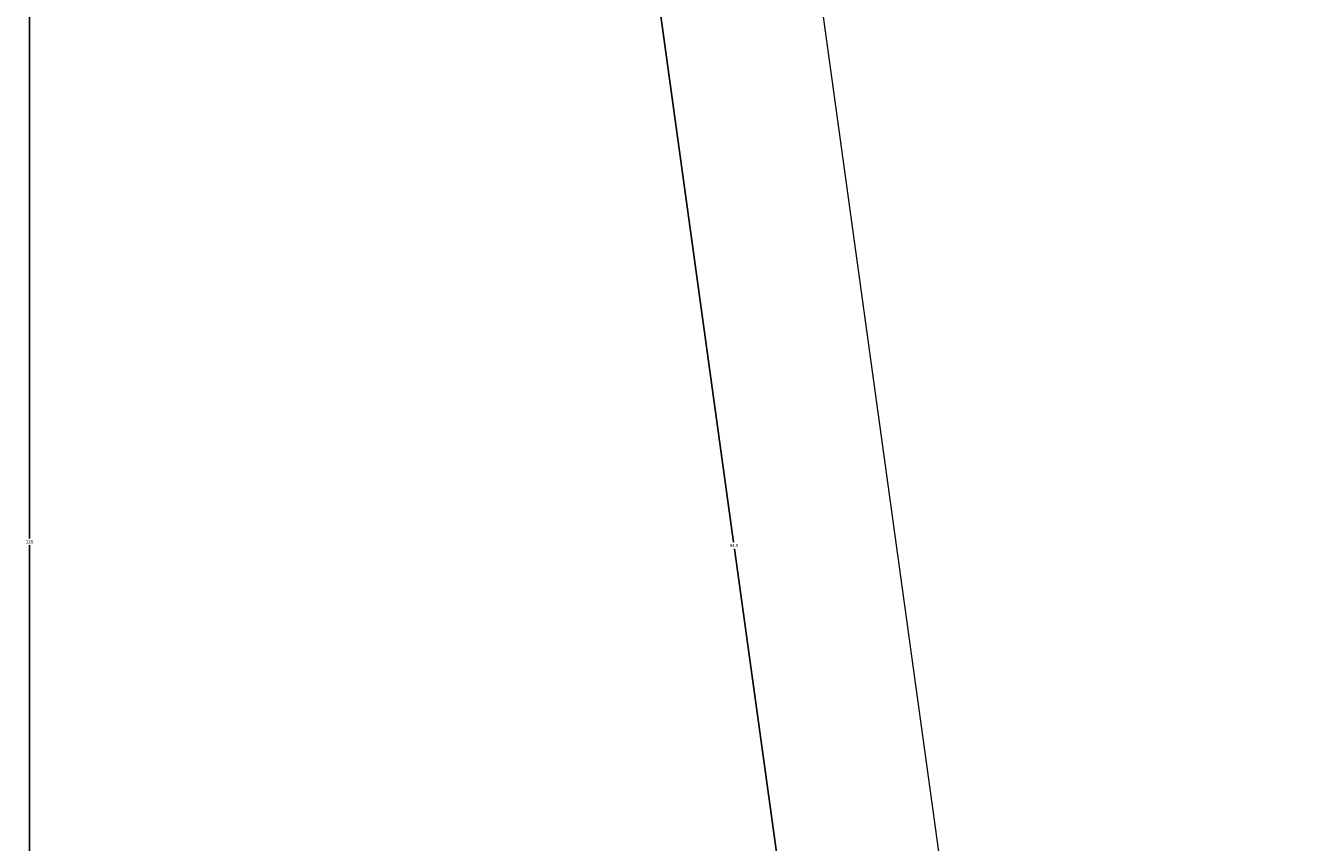
# Model space of a CAD drawing. Units: millimetres. Extents: x -9 to 135, y -119 to 27.
# Tile 3 of 12: x -9 to 62, y -63 to -18. Entities that reach past the tile are written whole.
import ezdxf

# ---------------------------------------------------------------- set-up
doc = ezdxf.new("R2010")
doc.units = ezdxf.units.MM
doc.layers.add('M-CONS', color=8, linetype='Continuous', lineweight=18)
doc.layers.add('M-DIMS', color=2, linetype='Continuous', lineweight=18)
doc.styles.get("Standard").update_dxf_attribs({"font": 'arial.ttf'})
doc.dimstyles.get("Standard").update_dxf_attribs({"dimtxt": 0.18, "dimasz": 0.18, "dimexe": 0.18, "dimexo": 0.0625, "dimgap": 0.09, "dimtad": 0, "dimtih": 1, "dimtoh": 1, "dimdec": 4, "dimzin": 0, "dimdsep": 46, "dimtxsty": 'Standard', "dimcen": 0.09, "dimadec": 0, "dimazin": 0, "dimtfac": 1, "dimtdec": 4, "dimtofl": 0, "dimtmove": 0, "dimatfit": 3, "dimfxl": 1, "dimtolj": 1, "dimtzin": 0, "dimarcsym": 0})

# ---------------------------------------------------------------- blocks, each defined once
blk = doc.blocks.new('*D3')
at = {"layer": 'Defpoints', "color": 0, "transparency": 16777216}
for p in [(0, 17.733), (-8.8, -110.267), (63, -110.267)]:
    blk.add_point(p, dxfattribs=at)
at = {"layer": 'M-DIMS', "color": 0, "lineweight": -2, "transparency": 16777216}
for p, q in [((-0.062, 17.733), (-8.98, 17.733)), ((-8.8, 17.553), (-8.8, -46.085)), ((-8.8, -110.087), (-8.8, -46.449)), ((62.938, -110.267), (-8.98, -110.267))]:
    blk.add_line(p, q, dxfattribs=at)
at = {"layer": 'M-DIMS', "color": 0, "transparency": 16777216}
for points in [[(-8.83, 17.553), (-8.77, 17.553), (-8.8, 17.733)], [(-8.83, -110.087), (-8.77, -110.087), (-8.8, -110.267)]]:
    blk.add_solid(points, dxfattribs=at)
at = {"layer": 'M-DIMS', "color": 0, "transparency": 16777216, "insert": (-8.8, -46.267), "char_height": 0.18, "attachment_point": 5}
blk.add_mtext('\\A1;128', dxfattribs=at)
blk = doc.blocks.new('*D14')
at = {"layer": 'Defpoints', "color": 0, "transparency": 16777216}
for p in [(32, 1.733), (23.283, 0.528), (45, -92.267)]:
    blk.add_point(p, dxfattribs=at)
at = {"layer": 'M-DIMS', "color": 0, "lineweight": -2, "transparency": 16777216}
for p, q in [((31.938, 1.725), (23.105, 0.503)), ((23.308, 0.349), (29.758, -46.29)), ((36.258, -93.294), (29.808, -46.654)), ((44.938, -92.275), (36.105, -93.497))]:
    blk.add_line(p, q, dxfattribs=at)
at = {"layer": 'M-DIMS', "color": 0, "transparency": 16777216}
for points in [[(23.337, 0.353), (23.278, 0.345), (23.283, 0.528)], [(36.288, -93.29), (36.229, -93.298), (36.283, -93.472)]]:
    blk.add_solid(points, dxfattribs=at)
at = {"layer": 'M-DIMS', "color": 0, "transparency": 16777216, "insert": (29.783, -46.472), "char_height": 0.18, "attachment_point": 5}
blk.add_mtext('\\A1;94.9', dxfattribs=at)

msp = doc.modelspace()

# ---------------------------------------------------------------- linework, layer by layer
at = {"layer": 'M-CONS'}
msp.add_line((32, 1.733, 115.129), (45, -92.267, 115.129), dxfattribs=at)

# ---------------------------------------------------------------- dimensions: what is measured, and where the dimension line sits
at = {"layer": 'M-DIMS'}
for base, p1, p2, angle, override, picture, middle in [((-8.8, -110.267), (0, 17.733), (63, -110.267), 90, {"dimdec": 0, "dimlfac": 1, "dimrnd": 0, "dimzin": 0, "dimdsep": 46, "dimlunit": 2}, '*D3', (-8.8, -46.267)), ((23.283, 0.528), (45, -92.267), (32, 1.733), 97.87394, {"dimdec": 1, "dimlfac": 1, "dimrnd": 0, "dimzin": 0, "dimdsep": 46, "dimlunit": 2}, '*D14', (29.783, -46.472))]:
    dim = msp.add_linear_dim(base=base, p1=p1, p2=p2, angle=angle, dimstyle='Standard', override=override, dxfattribs=at)
    dim.commit()
    dim.dimension.update_dxf_attribs({"geometry": picture, "text_midpoint": middle})

doc.saveas('drawing.dxf')
